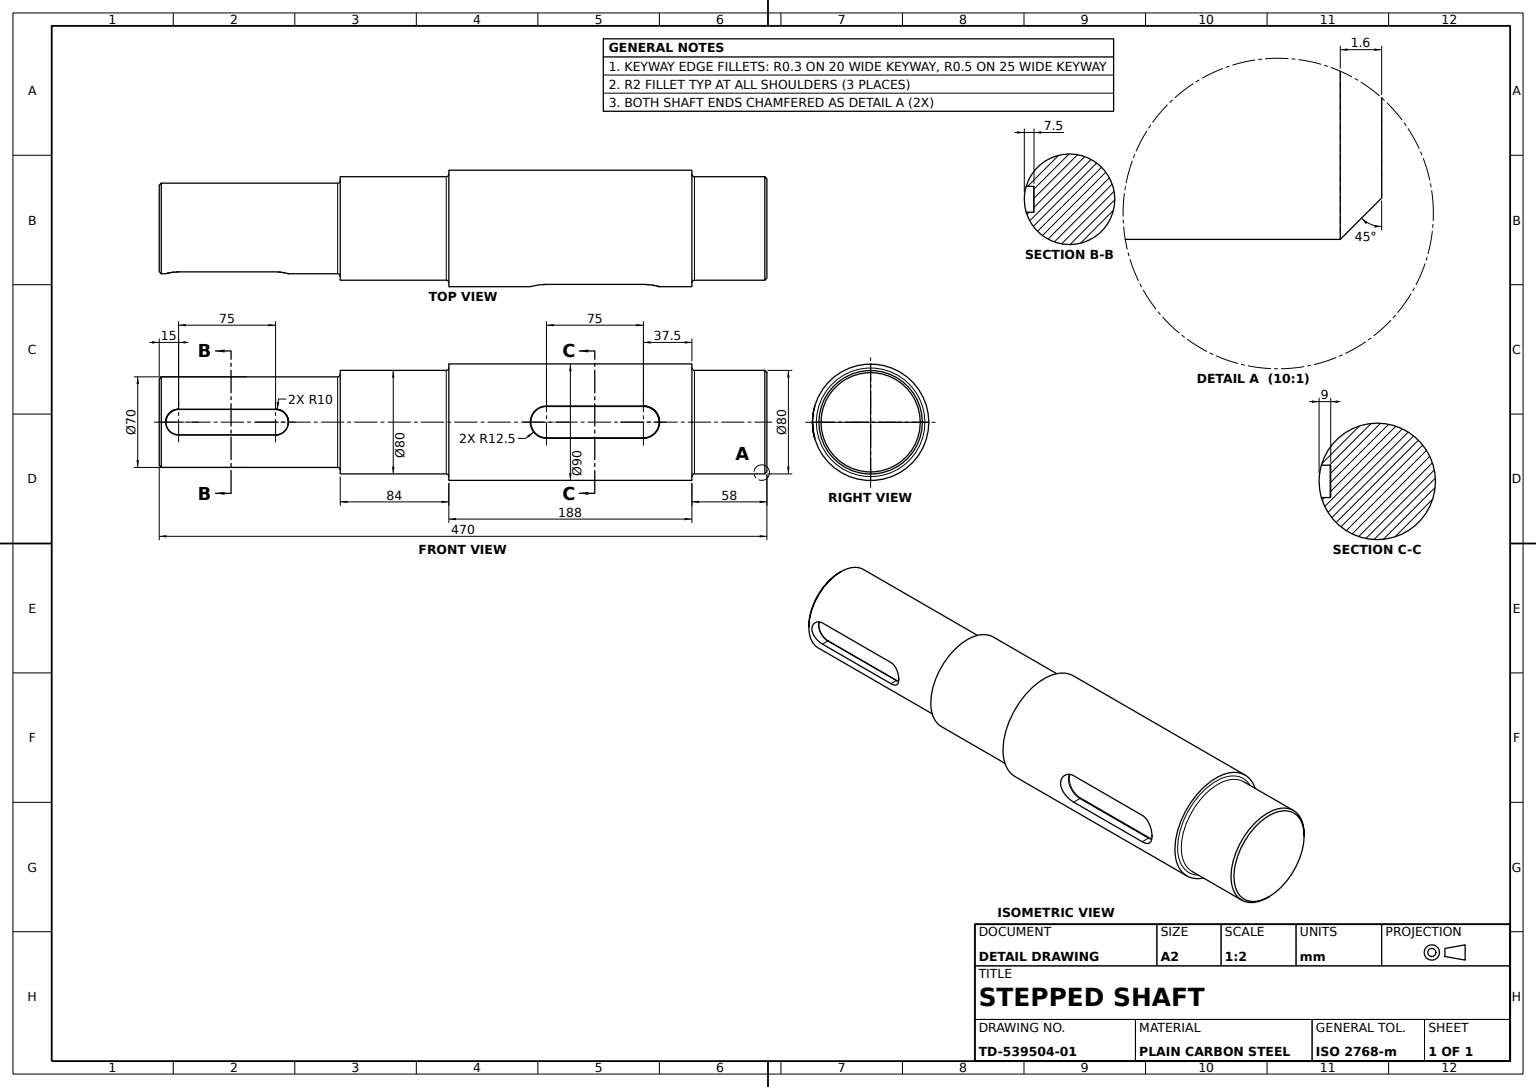
from build123d import *
from OCP.BRepFilletAPI import BRepFilletAPI_MakeFillet

# Parameters (mm, degrees)
END_CHAMFER_1_6X45_SIZE  = 1.6
SHOULDER_FILLETS_R2_R    = 2
KEYWAY_START             = 35
KEYWAY_1_DEPTH_7_5_DEPTH = 7.5
KEYWAY_START_2           = 45
KEYWAY_2_DEPTH_9_DEPTH   = 9
KEYWAY_EDGE_FILLETS_R1   = 0.3
KEYWAY_EDGE_FILLETS_R2   = 0.5


with BuildPart() as part:
    # Shaft Profile Sketch → Stepped Shaft Body (revolve)
    with BuildSketch(Plane(origin=(0, 0, 0), x_dir=(0, 0, -1), z_dir=(1, 0, 0)), mode=Mode.PRIVATE) as stepped_shaft_body_sk:
        Polygon((-224, 0), (-224, -35), (-84, -35), (-84, -40), (0, -40), (0, -45), (188, -45), (188, -40), (246, -40), (246, 0), align=None)
    revolve(stepped_shaft_body_sk.sketch.rotate(Axis((0, 0, 224), (0, 0, -1)), 270), axis=Axis((0, 0, 224), (0, 0, -1)))

    # End Chamfer 1.6x45
    end_chamfer_1_6x45_edges = [part.edges().sort_by_distance(p)[0] for p in [
        (-35, 0, 224),
        (-40, 0, -246),
    ]]
    chamfer(end_chamfer_1_6x45_edges, length=END_CHAMFER_1_6X45_SIZE)

    # Shoulder Fillets R2
    shoulder_fillets_r2_edges = [part.edges().sort_by_distance(p)[0] for p in [
        (-40, 0, 0),
        (-35, 0, 84),
        (-40, 0, -188),
    ]]
    fillet(shoulder_fillets_r2_edges, radius=SHOULDER_FILLETS_R2_R)

    # Keyway Slots Sketch → Keyway 1 Depth 7.5 (cut)
    with BuildSketch(Plane(origin=(0, 0, 0), x_dir=(0, 0, -1), z_dir=(1, 0, 0)).offset(KEYWAY_START)):
        with BuildLine():
            Line((-209, 10), (-134, 10))
            ThreePointArc((-134, 10), (-124, 0), (-134, -10))
            Line((-134, -10), (-209, -10))
            ThreePointArc((-209, -10), (-219, 0), (-209, 10))
        make_face()
    extrude(amount=-KEYWAY_1_DEPTH_7_5_DEPTH, mode=Mode.SUBTRACT)

    # Sketch2_3 → Keyway 2 Depth 9 (cut)
    with BuildSketch(Plane(origin=(0, 0, 0), x_dir=(0, 0, -1), z_dir=(1, 0, 0)).offset(KEYWAY_START_2)):
        with BuildLine():
            Line((75.5, 12.5), (150.5, 12.5))
            ThreePointArc((150.5, 12.5), (163, 0), (150.5, -12.5))
            Line((150.5, -12.5), (75.5, -12.5))
            ThreePointArc((75.5, -12.5), (63, 0), (75.5, 12.5))
        make_face()
    extrude(amount=-KEYWAY_2_DEPTH_9_DEPTH, mode=Mode.SUBTRACT)

    # Keyway Edge Fillets: one fillet with a radius per group of edges: ONE call of the kernel's fillet builder (fillet() takes one radius for all edges)
    keyway_edge_fillets_edges_1 = [part.edges().sort_by_distance(p)[0] for p in [
        (27.5, 0, 219),
        (27.5, 0, 124),
        (27.5, -10, 171.5),
        (27.5, 10, 171.5),
    ]]
    keyway_edge_fillets_edges_2 = [part.edges().sort_by_distance(p)[0] for p in [
        (36, 0, -163),
        (36, -12.5, -113),
        (36, 0, -63),
        (36, 12.5, -113),
    ]]
    keyway_edge_fillets = BRepFilletAPI_MakeFillet(part.part.solid().wrapped)
    for e in keyway_edge_fillets_edges_1:
        keyway_edge_fillets.Add(KEYWAY_EDGE_FILLETS_R1, e.wrapped)
    for e in keyway_edge_fillets_edges_2:
        keyway_edge_fillets.Add(KEYWAY_EDGE_FILLETS_R2, e.wrapped)
    add(Compound.cast(keyway_edge_fillets.Shape()), mode=Mode.REPLACE)


solid = part.part
